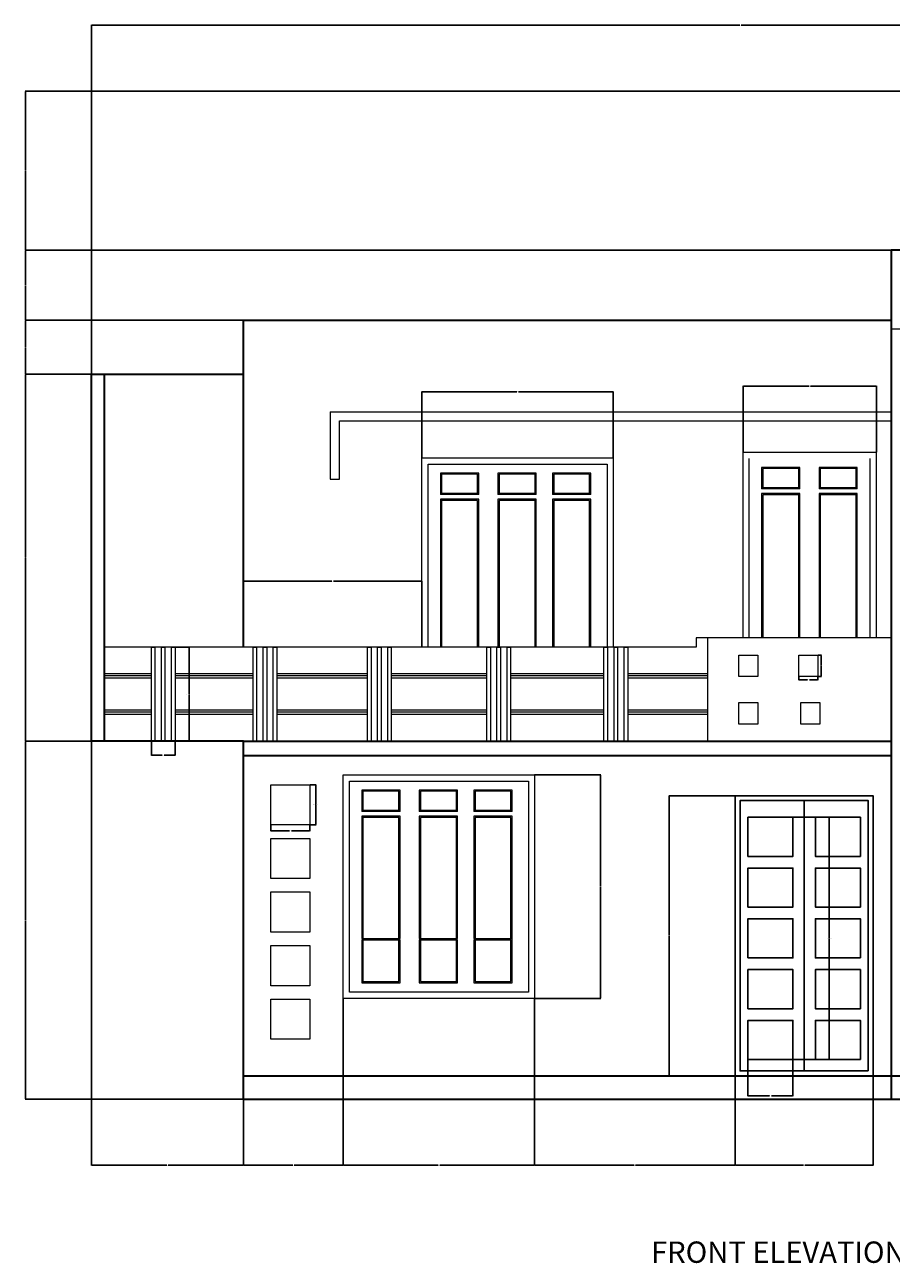
# Model space of a CAD drawing. Units: inches. Extents: x 1741 to 3812, y 9290 to 10023.
# Tile 4 of 5: x 3008 to 3495, y 9327 to 10023. Entities that reach past the tile are written whole.
import ezdxf

# ---------------------------------------------------------------- set-up
doc = ezdxf.new("R2010")
doc.units = ezdxf.units.IN
doc.header["$MEASUREMENT"] = 0
for name, color, linetype, lineweight in [('A-ANNO-DIMS', 2, 'Continuous', 18), ('A-ANNO-TEXT', 7, 'Continuous', 25), ('A-DOOR-ELEV', 3, 'Continuous', 25), ('A-ELEV', 7, 'Continuous', 35), ('A-ELEV-RAIL', 3, 'Continuous', 18), ('A-ELEV-TRIM', 9, 'Continuous', 18), ('A-GLAZ-ELEV', 4, 'Continuous', 18)]:
    doc.layers.add(name, color=color, linetype=linetype, lineweight=lineweight)
doc.styles.get("Standard").update_dxf_attribs({"font": 'arial.ttf'})
doc.dimstyles.get("Standard").update_dxf_attribs({"dimtxt": 0.18, "dimasz": 0.18, "dimexe": 0.18, "dimexo": 0.0625, "dimgap": 0.09, "dimtad": 0, "dimtih": 1, "dimtoh": 1, "dimdec": 4, "dimzin": 0, "dimdsep": 46, "dimtxsty": 'Standard', "dimcen": 0.09, "dimadec": 0, "dimazin": 0, "dimtfac": 1, "dimtdec": 4, "dimtofl": 0, "dimtmove": 0, "dimatfit": 3, "dimfxl": 1, "dimtolj": 1, "dimtzin": 0, "dimarcsym": 0})

# ---------------------------------------------------------------- blocks, each defined once
blk = doc.blocks.new('GLAZ-TRANSOM-LIGHT')
for p, q in [((0, 12.07), (0, 0)), ((21.51, 12.07), (0, 12.07)), ((0.66, 11.41), (0.66, 0.66)), ((20.85, 11.41), (0.66, 11.41)), ((20.85, 0.66), (20.85, 11.41)), ((21.51, 0), (21.51, 12.07)), ((20.85, 0.66), (0.66, 0.66)), ((21.51, 0), (0, 0))]:
    blk.add_line(p, q)
blk = doc.blocks.new('DOOR-LEAF-PANEL-SET')
for points in [[(0, 114.23), (25.3, 114.23), (25.3, 136.25), (0, 136.25)], [(0, 85.68), (25.3, 85.68), (25.3, 107.69), (0, 107.69)], [(0, 57.12), (25.3, 57.12), (25.3, 79.13), (0, 79.13)], [(0, 28.56), (25.3, 28.56), (25.3, 50.57), (0, 50.57)], [(0, 0), (25.3, 0), (25.3, 22.01), (0, 22.01)]]:
    blk.add_lwpolyline(points, close=True)
blk = doc.blocks.new('BALCONY-RAIL-POST-CLUSTER')
for points in [[(0, 52.73), (1.96, 52.73), (1.96, 0), (0, 0)], [(5.66, 52.73), (7.63, 52.73), (7.63, 0), (5.66, 0)], [(11.35, 52.73), (13.31, 52.73), (13.31, 0), (11.35, 0)]]:
    blk.add_lwpolyline(points, close=True)
blk = doc.blocks.new('BALCONY-PARAPET-REVEAL')
blk.add_lwpolyline([(0, 12.07), (10.64, 12.07), (10.64, 0), (0, 0)], close=True)
blk = doc.blocks.new('FACADE-RECESSED-PANEL')
blk.add_lwpolyline([(0, 22.57), (21.93, 22.57), (21.93, 0), (0, 0)], close=True)
blk = doc.blocks.new('*D19')
at = {"layer": 'A-ANNO-DIMS', "color": 0, "lineweight": -2, "transparency": 16777216}
for p, q in [((3092.52, 9673.01), (3100.55, 9673.01)), ((3100.37, 9672.83), (3100.37, 9646.83)), ((3100.37, 9620.47), (3100.37, 9646.47)), ((3092.52, 9620.29), (3100.55, 9620.29))]:
    blk.add_line(p, q, dxfattribs=at)
at = {"layer": 'A-ANNO-DIMS', "color": 0, "transparency": 16777216}
for points in [[(3100.34, 9672.83), (3100.4, 9672.83), (3100.37, 9673.01)], [(3100.34, 9620.47), (3100.4, 9620.47), (3100.37, 9620.29)]]:
    blk.add_solid(points, dxfattribs=at)
at = {"layer": 'Defpoints', "color": 0, "transparency": 16777216}
for p in [(3092.46, 9673.01), (3100.37, 9673.01), (3092.46, 9620.29)]:
    blk.add_point(p, dxfattribs=at)
at = {"layer": 'A-ANNO-DIMS', "color": 0, "transparency": 16777216, "insert": (3100.37, 9646.65), "char_height": 0.18, "attachment_point": 5}
blk.add_mtext('\\A1;RAIL POST GROUP 53 TYP.', dxfattribs=at)
blk = doc.blocks.new('*D20')
at = {"layer": 'A-ANNO-DIMS', "color": 0, "lineweight": -2, "transparency": 16777216}
for p, q in [((3079.15, 9620.22), (3079.15, 9612.2)), ((3092.46, 9620.22), (3092.46, 9612.2)), ((3079.33, 9612.38), (3085.29, 9612.38)), ((3092.28, 9612.38), (3086.33, 9612.38))]:
    blk.add_line(p, q, dxfattribs=at)
at = {"layer": 'A-ANNO-DIMS', "color": 0, "transparency": 16777216}
for points in [[(3079.33, 9612.41), (3079.33, 9612.35), (3079.15, 9612.38)], [(3092.28, 9612.41), (3092.28, 9612.35), (3092.46, 9612.38)]]:
    blk.add_solid(points, dxfattribs=at)
at = {"layer": 'Defpoints', "color": 0, "transparency": 16777216}
for p in [(3079.15, 9620.29), (3092.46, 9620.29), (3092.46, 9612.38)]:
    blk.add_point(p, dxfattribs=at)
at = {"layer": 'A-ANNO-DIMS', "color": 0, "transparency": 16777216, "insert": (3085.81, 9612.38), "char_height": 0.18, "attachment_point": 5}
blk.add_mtext('\\A1;13 TYP.', dxfattribs=at)
blk = doc.blocks.new('*D23')
at = {"layer": 'A-ANNO-DIMS', "color": 0, "lineweight": -2, "transparency": 16777216}
for p, q in [((3168.33, 9595.77), (3171.83, 9595.77)), ((3171.65, 9595.59), (3171.65, 9584.67)), ((3171.65, 9573.38), (3171.65, 9584.3)), ((3168.33, 9573.2), (3171.83, 9573.2))]:
    blk.add_line(p, q, dxfattribs=at)
at = {"layer": 'A-ANNO-DIMS', "color": 0, "transparency": 16777216}
for points in [[(3171.62, 9595.59), (3171.68, 9595.59), (3171.65, 9595.77)], [(3171.62, 9573.38), (3171.68, 9573.38), (3171.65, 9573.2)]]:
    blk.add_solid(points, dxfattribs=at)
at = {"layer": 'Defpoints', "color": 0, "transparency": 16777216}
for p in [(3168.27, 9595.77), (3171.65, 9595.77), (3168.27, 9573.2)]:
    blk.add_point(p, dxfattribs=at)
at = {"layer": 'A-ANNO-DIMS', "color": 0, "transparency": 16777216, "insert": (3171.65, 9584.48), "char_height": 0.18, "attachment_point": 5}
blk.add_mtext('\\A1;RECESSED PANEL 23 TYP.', dxfattribs=at)
blk = doc.blocks.new('*D24')
at = {"layer": 'A-ANNO-DIMS', "color": 0, "lineweight": -2, "transparency": 16777216}
for p, q in [((3146.33, 9573.14), (3146.33, 9569.63)), ((3168.27, 9573.14), (3168.27, 9569.63)), ((3146.51, 9569.81), (3156.77, 9569.81)), ((3168.09, 9569.81), (3157.83, 9569.81))]:
    blk.add_line(p, q, dxfattribs=at)
at = {"layer": 'A-ANNO-DIMS', "color": 0, "transparency": 16777216}
for points in [[(3146.51, 9569.84), (3146.51, 9569.78), (3146.33, 9569.81)], [(3168.09, 9569.84), (3168.09, 9569.78), (3168.27, 9569.81)]]:
    blk.add_solid(points, dxfattribs=at)
at = {"layer": 'Defpoints', "color": 0, "transparency": 16777216}
for p in [(3146.33, 9573.2), (3168.27, 9573.2), (3168.27, 9569.81)]:
    blk.add_point(p, dxfattribs=at)
at = {"layer": 'A-ANNO-DIMS', "color": 0, "transparency": 16777216, "insert": (3157.3, 9569.81), "char_height": 0.18, "attachment_point": 5}
blk.add_mtext('\\A1;22 TYP.', dxfattribs=at)
blk = doc.blocks.new('*D25')
at = {"layer": 'A-ANNO-DIMS', "color": 0, "lineweight": -2, "transparency": 16777216}
for p, q in [((3453.73, 9668.66), (3455.66, 9668.66)), ((3455.48, 9668.48), (3455.48, 9662.81)), ((3455.48, 9656.78), (3455.48, 9662.45)), ((3453.73, 9656.6), (3455.66, 9656.6))]:
    blk.add_line(p, q, dxfattribs=at)
at = {"layer": 'A-ANNO-DIMS', "color": 0, "transparency": 16777216}
for points in [[(3455.45, 9668.48), (3455.51, 9668.48), (3455.48, 9668.66)], [(3455.45, 9656.78), (3455.51, 9656.78), (3455.48, 9656.6)]]:
    blk.add_solid(points, dxfattribs=at)
at = {"layer": 'Defpoints', "color": 0, "transparency": 16777216}
for p in [(3453.67, 9668.66), (3455.48, 9668.66), (3453.67, 9656.6)]:
    blk.add_point(p, dxfattribs=at)
at = {"layer": 'A-ANNO-DIMS', "color": 0, "transparency": 16777216, "insert": (3455.48, 9662.63), "char_height": 0.18, "attachment_point": 5}
blk.add_mtext('\\A1;BALCONY REVEAL 12 TYP.', dxfattribs=at)
blk = doc.blocks.new('*D26')
at = {"layer": 'A-ANNO-DIMS', "color": 0, "lineweight": -2, "transparency": 16777216}
for p, q in [((3443.02, 9656.54), (3443.02, 9654.61)), ((3453.67, 9656.54), (3453.67, 9654.61)), ((3443.2, 9654.79), (3447.82, 9654.79)), ((3453.49, 9654.79), (3448.86, 9654.79))]:
    blk.add_line(p, q, dxfattribs=at)
at = {"layer": 'A-ANNO-DIMS', "color": 0, "transparency": 16777216}
for points in [[(3443.2, 9654.82), (3443.2, 9654.76), (3443.02, 9654.79)], [(3453.49, 9654.82), (3453.49, 9654.76), (3453.67, 9654.79)]]:
    blk.add_solid(points, dxfattribs=at)
at = {"layer": 'Defpoints', "color": 0, "transparency": 16777216}
for p in [(3443.02, 9656.6), (3453.67, 9656.6), (3453.67, 9654.79)]:
    blk.add_point(p, dxfattribs=at)
at = {"layer": 'A-ANNO-DIMS', "color": 0, "transparency": 16777216, "insert": (3448.34, 9654.79), "char_height": 0.18, "attachment_point": 5}
blk.add_mtext('\\A1;11 TYP.', dxfattribs=at)
blk = doc.blocks.new('*D29')
at = {"layer": 'A-ANNO-DIMS', "color": 0, "lineweight": -2, "transparency": 16777216}
for p, q in [((3439.68, 9577.53), (3460.23, 9577.53)), ((3460.05, 9577.35), (3460.05, 9509.59)), ((3460.05, 9441.46), (3460.05, 9509.22)), ((3439.68, 9441.28), (3460.23, 9441.28))]:
    blk.add_line(p, q, dxfattribs=at)
at = {"layer": 'A-ANNO-DIMS', "color": 0, "transparency": 16777216}
for points in [[(3460.02, 9577.35), (3460.08, 9577.35), (3460.05, 9577.53)], [(3460.02, 9441.46), (3460.08, 9441.46), (3460.05, 9441.28)]]:
    blk.add_solid(points, dxfattribs=at)
at = {"layer": 'Defpoints', "color": 0, "transparency": 16777216}
for p in [(3439.61, 9577.53), (3460.05, 9577.53), (3439.61, 9441.28)]:
    blk.add_point(p, dxfattribs=at)
at = {"layer": 'A-ANNO-DIMS', "color": 0, "transparency": 16777216, "insert": (3460.05, 9509.41), "char_height": 0.18, "attachment_point": 5}
blk.add_mtext('\\A1;LEAF PANELS 136 TYP.', dxfattribs=at)
blk = doc.blocks.new('*D30')
at = {"layer": 'A-ANNO-DIMS', "color": 0, "lineweight": -2, "transparency": 16777216}
for p, q in [((3414.31, 9441.22), (3414.31, 9420.66)), ((3439.61, 9441.22), (3439.61, 9420.66)), ((3414.49, 9420.84), (3426.43, 9420.84)), ((3439.43, 9420.84), (3427.49, 9420.84))]:
    blk.add_line(p, q, dxfattribs=at)
at = {"layer": 'A-ANNO-DIMS', "color": 0, "transparency": 16777216}
for points in [[(3414.49, 9420.87), (3414.49, 9420.81), (3414.31, 9420.84)], [(3439.43, 9420.87), (3439.43, 9420.81), (3439.61, 9420.84)]]:
    blk.add_solid(points, dxfattribs=at)
at = {"layer": 'Defpoints', "color": 0, "transparency": 16777216}
for p in [(3414.31, 9441.28), (3439.61, 9441.28), (3439.61, 9420.84)]:
    blk.add_point(p, dxfattribs=at)
at = {"layer": 'A-ANNO-DIMS', "color": 0, "transparency": 16777216, "insert": (3426.96, 9420.84), "char_height": 0.18, "attachment_point": 5}
blk.add_mtext('\\A1;25 TYP.', dxfattribs=at)
blk = doc.blocks.new('*D77')
at = {"layer": 'A-ANNO-DIMS', "color": 0, "lineweight": -2, "transparency": 16777216}
for p, q in [((3045.51, 9826.55), (3045.51, 10022.94)), ((3045.69, 10022.76), (3409.82, 10022.76)), ((3774.74, 10022.76), (3410.61, 10022.76)), ((3774.92, 9985.72), (3774.92, 10022.94))]:
    blk.add_line(p, q, dxfattribs=at)
at = {"layer": 'A-ANNO-DIMS', "color": 0, "transparency": 16777216}
for points in [[(3045.69, 10022.79), (3045.69, 10022.73), (3045.51, 10022.76)], [(3774.74, 10022.79), (3774.74, 10022.73), (3774.92, 10022.76)]]:
    blk.add_solid(points, dxfattribs=at)
at = {"layer": 'Defpoints', "color": 0, "transparency": 16777216}
for p in [(3774.92, 10022.76), (3774.92, 9985.66), (3045.51, 9826.49)]:
    blk.add_point(p, dxfattribs=at)
at = {"layer": 'A-ANNO-DIMS', "color": 0, "transparency": 16777216, "insert": (3410.21, 10022.76), "char_height": 0.18, "attachment_point": 5}
blk.add_mtext('\\A1;729.4', dxfattribs=at)
blk = doc.blocks.new('*D79')
at = {"layer": 'A-ANNO-DIMS', "color": 0, "lineweight": -2, "transparency": 16777216}
for p, q in [((3045.51, 9620.22), (3045.51, 9381.78)), ((3130.92, 9419), (3130.92, 9381.78)), ((3045.69, 9381.96), (3087.89, 9381.96)), ((3130.74, 9381.96), (3088.54, 9381.96))]:
    blk.add_line(p, q, dxfattribs=at)
at = {"layer": 'A-ANNO-DIMS', "color": 0, "transparency": 16777216}
for points in [[(3045.69, 9381.99), (3045.69, 9381.93), (3045.51, 9381.96)], [(3130.74, 9381.99), (3130.74, 9381.93), (3130.92, 9381.96)]]:
    blk.add_solid(points, dxfattribs=at)
at = {"layer": 'Defpoints', "color": 0, "transparency": 16777216}
for p in [(3045.51, 9620.29), (3130.92, 9419.06), (3130.92, 9381.96)]:
    blk.add_point(p, dxfattribs=at)
at = {"layer": 'A-ANNO-DIMS', "color": 0, "transparency": 16777216, "insert": (3088.22, 9381.96), "char_height": 0.18, "attachment_point": 5}
blk.add_mtext('\\A1;85.4', dxfattribs=at)
blk = doc.blocks.new('*D80')
at = {"layer": 'A-ANNO-DIMS', "color": 0, "lineweight": -2, "transparency": 16777216}
for p, q in [((3186.98, 9475.64), (3186.98, 9381.78)), ((3130.92, 9419), (3130.92, 9381.78)), ((3131.1, 9381.96), (3158.56, 9381.96)), ((3186.8, 9381.96), (3159.34, 9381.96))]:
    blk.add_line(p, q, dxfattribs=at)
at = {"layer": 'A-ANNO-DIMS', "color": 0, "transparency": 16777216}
for points in [[(3131.1, 9381.99), (3131.1, 9381.93), (3130.92, 9381.96)], [(3186.8, 9381.99), (3186.8, 9381.93), (3186.98, 9381.96)]]:
    blk.add_solid(points, dxfattribs=at)
at = {"layer": 'Defpoints', "color": 0, "transparency": 16777216}
for p in [(3186.98, 9475.7), (3130.92, 9419.06), (3186.98, 9381.96)]:
    blk.add_point(p, dxfattribs=at)
at = {"layer": 'A-ANNO-DIMS', "color": 0, "transparency": 16777216, "insert": (3158.95, 9381.96), "char_height": 0.18, "attachment_point": 5}
blk.add_mtext('\\A1;56.07', dxfattribs=at)
blk = doc.blocks.new('*D81')
at = {"layer": 'A-ANNO-DIMS', "color": 0, "lineweight": -2, "transparency": 16777216}
for p, q in [((3186.98, 9475.64), (3186.98, 9381.78)), ((3294.43, 9475.64), (3294.43, 9381.78)), ((3187.16, 9381.96), (3240.25, 9381.96)), ((3294.25, 9381.96), (3241.16, 9381.96))]:
    blk.add_line(p, q, dxfattribs=at)
at = {"layer": 'A-ANNO-DIMS', "color": 0, "transparency": 16777216}
for points in [[(3187.16, 9381.99), (3187.16, 9381.93), (3186.98, 9381.96)], [(3294.25, 9381.99), (3294.25, 9381.93), (3294.43, 9381.96)]]:
    blk.add_solid(points, dxfattribs=at)
at = {"layer": 'Defpoints', "color": 0, "transparency": 16777216}
for p in [(3186.98, 9475.7), (3294.43, 9475.7), (3294.43, 9381.96)]:
    blk.add_point(p, dxfattribs=at)
at = {"layer": 'A-ANNO-DIMS', "color": 0, "transparency": 16777216, "insert": (3240.71, 9381.96), "char_height": 0.18, "attachment_point": 5}
blk.add_mtext('\\A1;107.44', dxfattribs=at)
blk = doc.blocks.new('*D82')
at = {"layer": 'A-ANNO-DIMS', "color": 0, "lineweight": -2, "transparency": 16777216}
for p, q in [((3294.43, 9475.64), (3294.43, 9381.78)), ((3407.19, 9432.13), (3407.19, 9381.78)), ((3294.61, 9381.96), (3350.35, 9381.96)), ((3407.01, 9381.96), (3351.26, 9381.96))]:
    blk.add_line(p, q, dxfattribs=at)
at = {"layer": 'A-ANNO-DIMS', "color": 0, "transparency": 16777216}
for points in [[(3294.61, 9381.99), (3294.61, 9381.93), (3294.43, 9381.96)], [(3407.01, 9381.99), (3407.01, 9381.93), (3407.19, 9381.96)]]:
    blk.add_solid(points, dxfattribs=at)
at = {"layer": 'Defpoints', "color": 0, "transparency": 16777216}
for p in [(3294.43, 9475.7), (3407.19, 9432.19), (3407.19, 9381.96)]:
    blk.add_point(p, dxfattribs=at)
at = {"layer": 'A-ANNO-DIMS', "color": 0, "transparency": 16777216, "insert": (3350.81, 9381.96), "char_height": 0.18, "attachment_point": 5}
blk.add_mtext('\\A1;112.76', dxfattribs=at)
blk = doc.blocks.new('*D83')
at = {"layer": 'A-ANNO-DIMS', "color": 0, "lineweight": -2, "transparency": 16777216}
for p, q in [((3407.19, 9432.13), (3407.19, 9381.78)), ((3484.64, 9432.13), (3484.64, 9381.78)), ((3407.37, 9381.96), (3445.52, 9381.96)), ((3484.46, 9381.96), (3446.31, 9381.96))]:
    blk.add_line(p, q, dxfattribs=at)
at = {"layer": 'A-ANNO-DIMS', "color": 0, "transparency": 16777216}
for points in [[(3407.37, 9381.99), (3407.37, 9381.93), (3407.19, 9381.96)], [(3484.46, 9381.99), (3484.46, 9381.93), (3484.64, 9381.96)]]:
    blk.add_solid(points, dxfattribs=at)
at = {"layer": 'Defpoints', "color": 0, "transparency": 16777216}
for p in [(3407.19, 9432.19), (3484.64, 9432.19), (3484.64, 9381.96)]:
    blk.add_point(p, dxfattribs=at)
at = {"layer": 'A-ANNO-DIMS', "color": 0, "transparency": 16777216, "insert": (3445.92, 9381.96), "char_height": 0.18, "attachment_point": 5}
blk.add_mtext('\\A1;77.46', dxfattribs=at)
blk = doc.blocks.new('*D87')
at = {"layer": 'A-ANNO-DIMS', "color": 0, "lineweight": -2, "transparency": 16777216}
for p, q in [((3130.86, 9620.29), (3008.23, 9620.29)), ((3008.41, 9620.11), (3008.41, 9519.86)), ((3008.41, 9419.24), (3008.41, 9519.49)), ((3130.86, 9419.06), (3008.23, 9419.06))]:
    blk.add_line(p, q, dxfattribs=at)
at = {"layer": 'A-ANNO-DIMS', "color": 0, "transparency": 16777216}
for points in [[(3008.38, 9620.11), (3008.44, 9620.11), (3008.41, 9620.29)], [(3008.38, 9419.24), (3008.44, 9419.24), (3008.41, 9419.06)]]:
    blk.add_solid(points, dxfattribs=at)
at = {"layer": 'Defpoints', "color": 0, "transparency": 16777216}
for p in [(3008.41, 9620.29), (3130.92, 9620.29), (3130.92, 9419.06)]:
    blk.add_point(p, dxfattribs=at)
at = {"layer": 'A-ANNO-DIMS', "color": 0, "transparency": 16777216, "insert": (3008.41, 9519.67), "char_height": 0.18, "attachment_point": 5}
blk.add_mtext('\\A1;201.23', dxfattribs=at)
blk = doc.blocks.new('*D88')
at = {"layer": 'A-ANNO-DIMS', "color": 0, "lineweight": -2, "transparency": 16777216}
for p, q in [((3045.45, 9826.49), (3008.23, 9826.49)), ((3008.41, 9826.31), (3008.41, 9723.57)), ((3008.41, 9620.47), (3008.41, 9723.21)), ((3045.45, 9620.29), (3008.23, 9620.29))]:
    blk.add_line(p, q, dxfattribs=at)
at = {"layer": 'A-ANNO-DIMS', "color": 0, "transparency": 16777216}
for points in [[(3008.38, 9826.31), (3008.44, 9826.31), (3008.41, 9826.49)], [(3008.38, 9620.47), (3008.44, 9620.47), (3008.41, 9620.29)]]:
    blk.add_solid(points, dxfattribs=at)
at = {"layer": 'Defpoints', "color": 0, "transparency": 16777216}
for p in [(3008.41, 9826.49), (3045.51, 9826.49), (3045.51, 9620.29)]:
    blk.add_point(p, dxfattribs=at)
at = {"layer": 'A-ANNO-DIMS', "color": 0, "transparency": 16777216, "insert": (3008.41, 9723.39), "char_height": 0.18, "attachment_point": 5}
blk.add_mtext('\\A1;206.2', dxfattribs=at)
blk = doc.blocks.new('*D89')
at = {"layer": 'A-ANNO-DIMS', "color": 0, "lineweight": -2, "transparency": 16777216}
for p, q in [((3130.86, 9856.96), (3008.23, 9856.96)), ((3008.41, 9856.78), (3008.41, 9841.91)), ((3008.41, 9826.67), (3008.41, 9841.54)), ((3045.45, 9826.49), (3008.23, 9826.49))]:
    blk.add_line(p, q, dxfattribs=at)
at = {"layer": 'A-ANNO-DIMS', "color": 0, "transparency": 16777216}
for points in [[(3008.38, 9856.78), (3008.44, 9856.78), (3008.41, 9856.96)], [(3008.38, 9826.67), (3008.44, 9826.67), (3008.41, 9826.49)]]:
    blk.add_solid(points, dxfattribs=at)
at = {"layer": 'Defpoints', "color": 0, "transparency": 16777216}
for p in [(3008.41, 9856.96), (3130.92, 9856.96), (3045.51, 9826.49)]:
    blk.add_point(p, dxfattribs=at)
at = {"layer": 'A-ANNO-DIMS', "color": 0, "transparency": 16777216, "insert": (3008.41, 9841.73), "char_height": 0.18, "attachment_point": 5}
blk.add_mtext('\\A1;30.47', dxfattribs=at)
blk = doc.blocks.new('*D90')
at = {"layer": 'A-ANNO-DIMS', "color": 0, "lineweight": -2, "transparency": 16777216}
for p, q in [((3494.79, 9896.18), (3008.23, 9896.18)), ((3008.41, 9896), (3008.41, 9876.75)), ((3008.41, 9857.14), (3008.41, 9876.39)), ((3130.86, 9856.96), (3008.23, 9856.96))]:
    blk.add_line(p, q, dxfattribs=at)
at = {"layer": 'A-ANNO-DIMS', "color": 0, "transparency": 16777216}
for points in [[(3008.38, 9896), (3008.44, 9896), (3008.41, 9896.18)], [(3008.38, 9857.14), (3008.44, 9857.14), (3008.41, 9856.96)]]:
    blk.add_solid(points, dxfattribs=at)
at = {"layer": 'Defpoints', "color": 0, "transparency": 16777216}
for p in [(3008.41, 9896.18), (3494.85, 9896.18), (3130.92, 9856.96)]:
    blk.add_point(p, dxfattribs=at)
at = {"layer": 'A-ANNO-DIMS', "color": 0, "transparency": 16777216, "insert": (3008.41, 9876.57), "char_height": 0.18, "attachment_point": 5}
blk.add_mtext('\\A1;39.22', dxfattribs=at)
blk = doc.blocks.new('*D91')
at = {"layer": 'A-ANNO-DIMS', "color": 0, "lineweight": -2, "transparency": 16777216}
for p, q in [((3580.43, 9985.66), (3008.23, 9985.66)), ((3008.41, 9985.48), (3008.41, 9941.1)), ((3008.41, 9896.36), (3008.41, 9940.74)), ((3494.79, 9896.18), (3008.23, 9896.18))]:
    blk.add_line(p, q, dxfattribs=at)
at = {"layer": 'A-ANNO-DIMS', "color": 0, "transparency": 16777216}
for points in [[(3008.38, 9985.48), (3008.44, 9985.48), (3008.41, 9985.66)], [(3008.38, 9896.36), (3008.44, 9896.36), (3008.41, 9896.18)]]:
    blk.add_solid(points, dxfattribs=at)
at = {"layer": 'Defpoints', "color": 0, "transparency": 16777216}
for p in [(3008.41, 9985.66), (3580.49, 9985.66), (3494.85, 9896.18)]:
    blk.add_point(p, dxfattribs=at)
at = {"layer": 'A-ANNO-DIMS', "color": 0, "transparency": 16777216, "insert": (3008.41, 9940.92), "char_height": 0.18, "attachment_point": 5}
blk.add_mtext('\\A1;89.48', dxfattribs=at)
blk = doc.blocks.new('*D94')
at = {"layer": 'A-ANNO-DIMS', "color": 0, "lineweight": -2, "transparency": 16777216}
for p, q in [((3294.49, 9601.3), (3331.71, 9601.3)), ((3331.53, 9601.12), (3331.53, 9538.68)), ((3331.53, 9475.88), (3331.53, 9538.32)), ((3294.49, 9475.7), (3331.71, 9475.7))]:
    blk.add_line(p, q, dxfattribs=at)
at = {"layer": 'A-ANNO-DIMS', "color": 0, "transparency": 16777216}
for points in [[(3331.5, 9601.12), (3331.56, 9601.12), (3331.53, 9601.3)], [(3331.5, 9475.88), (3331.56, 9475.88), (3331.53, 9475.7)]]:
    blk.add_solid(points, dxfattribs=at)
at = {"layer": 'Defpoints', "color": 0, "transparency": 16777216}
for p in [(3294.43, 9601.3), (3294.43, 9475.7), (3331.53, 9475.7)]:
    blk.add_point(p, dxfattribs=at)
at = {"layer": 'A-ANNO-DIMS', "color": 0, "transparency": 16777216, "insert": (3331.53, 9538.5), "char_height": 0.18, "attachment_point": 5}
blk.add_mtext('\\A1;125.6', dxfattribs=at)
blk = doc.blocks.new('*D95')
at = {"layer": 'A-ANNO-DIMS', "color": 0, "lineweight": -2, "transparency": 16777216}
for p, q in [((3407.13, 9589.56), (3369.91, 9589.56)), ((3370.09, 9589.38), (3370.09, 9511.06)), ((3370.09, 9432.37), (3370.09, 9510.69)), ((3407.13, 9432.19), (3369.91, 9432.19))]:
    blk.add_line(p, q, dxfattribs=at)
at = {"layer": 'A-ANNO-DIMS', "color": 0, "transparency": 16777216}
for points in [[(3370.06, 9589.38), (3370.12, 9589.38), (3370.09, 9589.56)], [(3370.06, 9432.37), (3370.12, 9432.37), (3370.09, 9432.19)]]:
    blk.add_solid(points, dxfattribs=at)
at = {"layer": 'Defpoints', "color": 0, "transparency": 16777216}
for p in [(3370.09, 9589.56), (3407.19, 9589.56), (3407.19, 9432.19)]:
    blk.add_point(p, dxfattribs=at)
at = {"layer": 'A-ANNO-DIMS', "color": 0, "transparency": 16777216, "insert": (3370.09, 9510.87), "char_height": 0.18, "attachment_point": 5}
blk.add_mtext('\\A1;157.36', dxfattribs=at)
blk = doc.blocks.new('*D98')
at = {"layer": 'A-ANNO-DIMS', "color": 0, "lineweight": -2, "transparency": 16777216}
for p, q in [((3130.92, 9673.08), (3130.92, 9710.29)), ((3131.1, 9710.11), (3180.59, 9710.11)), ((3230.99, 9710.11), (3181.5, 9710.11)), ((3231.17, 9673.08), (3231.17, 9710.29))]:
    blk.add_line(p, q, dxfattribs=at)
at = {"layer": 'A-ANNO-DIMS', "color": 0, "transparency": 16777216}
for points in [[(3131.1, 9710.14), (3131.1, 9710.08), (3130.92, 9710.11)], [(3230.99, 9710.14), (3230.99, 9710.08), (3231.17, 9710.11)]]:
    blk.add_solid(points, dxfattribs=at)
at = {"layer": 'Defpoints', "color": 0, "transparency": 16777216}
for p in [(3231.17, 9710.11), (3130.92, 9673.01), (3231.17, 9673.01)]:
    blk.add_point(p, dxfattribs=at)
at = {"layer": 'A-ANNO-DIMS', "color": 0, "transparency": 16777216, "insert": (3181.05, 9710.11), "char_height": 0.18, "attachment_point": 5}
blk.add_mtext('\\A1;100.25', dxfattribs=at)
blk = doc.blocks.new('*D99')
at = {"layer": 'A-ANNO-DIMS', "color": 0, "lineweight": -2, "transparency": 16777216}
for p, q in [((3231.17, 9779.53), (3231.17, 9816.75)), ((3231.35, 9816.57), (3284.44, 9816.57)), ((3338.44, 9816.57), (3285.35, 9816.57)), ((3338.62, 9779.53), (3338.62, 9816.75))]:
    blk.add_line(p, q, dxfattribs=at)
at = {"layer": 'A-ANNO-DIMS', "color": 0, "transparency": 16777216}
for points in [[(3231.35, 9816.6), (3231.35, 9816.54), (3231.17, 9816.57)], [(3338.44, 9816.6), (3338.44, 9816.54), (3338.62, 9816.57)]]:
    blk.add_solid(points, dxfattribs=at)
at = {"layer": 'Defpoints', "color": 0, "transparency": 16777216}
for p in [(3338.62, 9816.57), (3231.17, 9779.47), (3338.62, 9779.47)]:
    blk.add_point(p, dxfattribs=at)
at = {"layer": 'A-ANNO-DIMS', "color": 0, "transparency": 16777216, "insert": (3284.89, 9816.57), "char_height": 0.18, "attachment_point": 5}
blk.add_mtext('\\A1;107.44', dxfattribs=at)
blk = doc.blocks.new('*D100')
at = {"layer": 'A-ANNO-DIMS', "color": 0, "lineweight": -2, "transparency": 16777216}
for p, q in [((3411.6, 9782.71), (3411.6, 9819.93)), ((3411.78, 9819.75), (3448.68, 9819.75)), ((3486.36, 9819.75), (3449.47, 9819.75)), ((3486.54, 9782.71), (3486.54, 9819.93))]:
    blk.add_line(p, q, dxfattribs=at)
at = {"layer": 'A-ANNO-DIMS', "color": 0, "transparency": 16777216}
for points in [[(3411.78, 9819.78), (3411.78, 9819.72), (3411.6, 9819.75)], [(3486.36, 9819.78), (3486.36, 9819.72), (3486.54, 9819.75)]]:
    blk.add_solid(points, dxfattribs=at)
at = {"layer": 'Defpoints', "color": 0, "transparency": 16777216}
for p in [(3486.54, 9819.75), (3411.6, 9782.65), (3486.54, 9782.65)]:
    blk.add_point(p, dxfattribs=at)
at = {"layer": 'A-ANNO-DIMS', "color": 0, "transparency": 16777216, "insert": (3449.07, 9819.75), "char_height": 0.18, "attachment_point": 5}
blk.add_mtext('\\A1;74.94', dxfattribs=at)

msp = doc.modelspace()

# ---------------------------------------------------------------- linework, layer by layer
at = {"layer": 'A-DOOR-ELEV'}
msp.add_line((3445.916, 9434.8933), (3445.916, 9586.8566), dxfattribs=at)
for points in [[(3484.6443, 9432.1944), (3407.1877, 9432.1944), (3407.1877, 9589.5555), (3484.6443, 9589.5555)], [(3481.9454, 9434.8933), (3409.8866, 9434.8933), (3409.8866, 9586.8566), (3481.9454, 9586.8566)]]:
    msp.add_lwpolyline(points, close=True, dxfattribs=at)
at = {"layer": 'A-ELEV'}
for p, q in [((3774.9155, 9896.1797), (3494.8475, 9896.1797)), ((3494.8475, 9896.1797), (3494.8475, 9419.0599)), ((3130.9182, 9856.9629), (3494.8475, 9856.9629)), ((3130.9182, 9673.0135), (3130.9182, 9856.9629)), ((3045.5138, 9620.287), (3045.5138, 9826.4899)), ((3045.5138, 9826.4899), (3130.9182, 9826.4899)), ((3052.8477, 9620.287), (3052.8477, 9826.4899)), ((3130.9182, 9620.287), (3045.5138, 9620.287)), ((3130.9182, 9620.287), (3494.8475, 9620.287)), ((3130.9182, 9419.0599), (3130.9182, 9620.287)), ((3130.9182, 9612.1944), (3494.8475, 9612.1944)), ((3130.9182, 9432.1944), (3774.9155, 9432.1944)), ((3130.9182, 9419.0599), (3774.9155, 9419.0599))]:
    msp.add_line(p, q, dxfattribs=at)
at = {"layer": 'A-ELEV-RAIL'}
for p, q in [((3494.8475, 9678.3912), (3385.1873, 9678.3912)), ((3385.1873, 9678.3912), (3385.1873, 9673.0135)), ((3391.6128, 9678.3912), (3391.6128, 9620.287)), ((3385.1873, 9673.0135), (3052.8477, 9673.0135)), ((3052.8477, 9658.2536), (3079.1511, 9658.2536)), ((3052.8477, 9657.0864), (3079.1511, 9657.0864)), ((3052.8477, 9655.9193), (3079.1511, 9655.9193)), ((3092.4615, 9658.2536), (3136.3361, 9658.2536)), ((3092.4615, 9657.0864), (3136.3361, 9657.0864)), ((3092.4615, 9655.9193), (3136.3361, 9655.9193)), ((3149.6465, 9658.2536), (3200.6041, 9658.2536)), ((3149.6465, 9657.0864), (3200.6041, 9657.0864)), ((3149.6465, 9655.9193), (3200.6041, 9655.9193)), ((3213.9145, 9658.2536), (3267.6685, 9658.2536)), ((3213.9145, 9657.0864), (3267.6685, 9657.0864)), ((3213.9145, 9655.9193), (3267.6685, 9655.9193)), ((3280.9789, 9658.2536), (3333.461, 9658.2536)), ((3280.9789, 9657.0864), (3333.461, 9657.0864)), ((3280.9789, 9655.9193), (3333.461, 9655.9193)), ((3346.7714, 9658.2536), (3391.6128, 9658.2536)), ((3346.7714, 9657.0864), (3391.6128, 9657.0864)), ((3346.7714, 9655.9193), (3391.6128, 9655.9193)), ((3052.8477, 9637.8286), (3079.1511, 9637.8286)), ((3052.8477, 9636.6615), (3079.1511, 9636.6615)), ((3052.8477, 9635.4943), (3079.1511, 9635.4943)), ((3092.4615, 9637.8286), (3136.3361, 9637.8286)), ((3092.4615, 9636.6615), (3136.3361, 9636.6615)), ((3092.4615, 9635.4943), (3136.3361, 9635.4943)), ((3149.6465, 9637.8286), (3200.6041, 9637.8286)), ((3149.6465, 9636.6615), (3200.6041, 9636.6615)), ((3149.6465, 9635.4943), (3200.6041, 9635.4943)), ((3213.9145, 9637.8286), (3267.6685, 9637.8286)), ((3213.9145, 9636.6615), (3267.6685, 9636.6615)), ((3213.9145, 9635.4943), (3267.6685, 9635.4943)), ((3280.9789, 9637.8286), (3333.461, 9637.8286)), ((3280.9789, 9636.6615), (3333.461, 9636.6615)), ((3280.9789, 9635.4943), (3333.461, 9635.4943)), ((3346.7714, 9637.8286), (3391.6128, 9637.8286)), ((3346.7714, 9636.6615), (3391.6128, 9636.6615)), ((3346.7714, 9635.4943), (3391.6128, 9635.4943))]:
    msp.add_line(p, q, dxfattribs=at)
msp.add_lwpolyline([(3338.6172, 9620.287), (3231.1727, 9620.287)], dxfattribs=at)
at = {"layer": 'A-ELEV-TRIM'}
for p, q in [((3730.5782, 9851.7953), (3494.8475, 9851.7953)), ((3179.5944, 9805.3348), (3494.8475, 9805.3348)), ((3179.5944, 9805.3348), (3179.5944, 9767.4573)), ((3184.8682, 9800.287), (3494.8475, 9800.287)), ((3184.8682, 9767.4573), (3184.8682, 9800.287)), ((3179.5944, 9767.4573), (3184.8682, 9767.4573))]:
    msp.add_line(p, q, dxfattribs=at)
at = {"layer": 'A-GLAZ-ELEV'}
for p, q in [((3411.6009, 9782.6524), (3486.5446, 9782.6524)), ((3263.1033, 9756.2208), (3241.5898, 9756.2208)), ((3241.5898, 9756.2208), (3241.5898, 9673.0135)), ((3262.4415, 9755.5591), (3242.2515, 9755.5591)), ((3242.2515, 9755.5591), (3242.2515, 9673.0135)), ((3262.4415, 9673.0135), (3262.4415, 9755.5591)), ((3263.1033, 9673.0135), (3263.1033, 9756.2208)), ((3443.5315, 9759.4078), (3422.018, 9759.4078)), ((3422.018, 9759.4078), (3422.018, 9678.3912)), ((3442.8697, 9758.7461), (3422.6797, 9758.7461)), ((3422.6797, 9758.7461), (3422.6797, 9678.3912)), ((3442.8697, 9678.3912), (3442.8697, 9758.7461)), ((3443.5315, 9678.3912), (3443.5315, 9759.4078)), ((3218.9149, 9578.0555), (3197.4014, 9578.0555)), ((3197.4014, 9578.0555), (3197.4014, 9509.2975)), ((3218.2531, 9577.3937), (3198.0631, 9577.3937)), ((3198.0631, 9577.3937), (3198.0631, 9509.2975)), ((3218.2531, 9509.2975), (3218.2531, 9577.3937)), ((3218.9149, 9509.2975), (3218.9149, 9578.0555)), ((3197.4014, 9509.2975), (3218.9149, 9509.2975)), ((3229.6716, 9509.2975), (3251.1851, 9509.2975)), ((3260.3482, 9509.2975), (3281.8616, 9509.2975)), ((3197.4014, 9508.6357), (3218.9149, 9508.6357)), ((3197.4014, 9508.6357), (3197.4014, 9484.5013)), ((3198.0631, 9508.6357), (3198.0631, 9485.163)), ((3218.2531, 9485.163), (3218.2531, 9508.6357)), ((3218.9149, 9484.5013), (3218.9149, 9508.6357)), ((3229.6716, 9508.6357), (3251.1851, 9508.6357)), ((3260.3482, 9508.6357), (3281.1999, 9508.6357)), ((3197.4014, 9484.5013), (3218.9149, 9484.5013)), ((3198.0631, 9485.163), (3218.2531, 9485.163))]:
    msp.add_line(p, q, dxfattribs=at)
for points in [[(3411.6009, 9678.3912), (3411.6009, 9782.6524)], [(3486.5446, 9678.3912), (3486.5446, 9782.6524)], [(3231.1727, 9673.0135), (3231.1727, 9779.4654), (3338.6172, 9779.4654), (3338.6172, 9673.0135)], [(3234.609, 9673.0135), (3234.609, 9776.0292), (3335.181, 9776.0292), (3335.181, 9673.0135)], [(3415.0372, 9678.3912), (3415.0372, 9779.2162)], [(3483.1083, 9678.3912), (3483.1083, 9779.2162)], [(3295.3735, 9673.0135), (3295.3735, 9756.2208), (3273.86, 9756.2208), (3273.86, 9673.0135)], [(3294.7117, 9673.0135), (3294.7117, 9755.5591), (3274.5218, 9755.5591), (3274.5218, 9673.0135)], [(3326.05, 9673.0135), (3326.05, 9756.2208), (3304.5366, 9756.2208), (3304.5366, 9673.0135)], [(3325.3883, 9673.0135), (3325.3883, 9755.5591), (3305.1983, 9755.5591), (3305.1983, 9673.0135)], [(3475.8017, 9678.3912), (3475.8017, 9759.4078), (3454.2882, 9759.4078), (3454.2882, 9678.3912)], [(3475.1399, 9678.3912), (3475.1399, 9758.7461), (3454.95, 9758.7461), (3454.95, 9678.3912)], [(3251.1851, 9509.2975), (3251.1851, 9578.0555), (3229.6716, 9578.0555), (3229.6716, 9509.2975)], [(3250.5233, 9509.2975), (3250.5233, 9577.3937), (3230.3333, 9577.3937), (3230.3333, 9509.2975)], [(3260.3482, 9508.6357), (3260.3482, 9484.5013), (3281.8616, 9484.5013), (3281.8616, 9578.0555), (3260.3482, 9578.0555), (3260.3482, 9509.2975)], [(3281.1999, 9509.2975), (3281.1999, 9577.3937), (3261.0099, 9577.3937), (3261.0099, 9509.2975)], [(3229.6716, 9508.6357), (3229.6716, 9484.5013), (3251.1851, 9484.5013), (3251.1851, 9508.6357)], [(3230.3333, 9508.6357), (3230.3333, 9485.163), (3250.5233, 9485.163), (3250.5233, 9508.6357)], [(3261.0099, 9508.6357), (3261.0099, 9485.163), (3281.1999, 9485.163), (3281.1999, 9508.6357)]]:
    msp.add_lwpolyline(points, dxfattribs=at)
for points in [[(3186.9843, 9601.3001), (3294.4288, 9601.3001), (3294.4288, 9475.7043), (3186.9843, 9475.7043)], [(3190.4206, 9597.8638), (3290.9926, 9597.8638), (3290.9926, 9479.1406), (3190.4206, 9479.1406)]]:
    msp.add_lwpolyline(points, close=True, dxfattribs=at)

# ---------------------------------------------------------------- block references
at = {"layer": 'A-DOOR-ELEV'}
msp.add_blockref('DOOR-LEAF-PANEL-SET', (3414.309, 9441.282), dxfattribs=at)
at = {"layer": 'A-DOOR-ELEV', "extrusion": (0, 0, -1), "zscale": -1}
msp.add_blockref('DOOR-LEAF-PANEL-SET', (-3477.523, 9441.282), dxfattribs=at)
at = {"layer": 'A-ELEV-RAIL'}
for p in [(3079.151, 9620.287), (3136.336, 9620.287), (3200.6039, 9620.287), (3267.6684, 9620.287), (3333.4609, 9620.287)]:
    msp.add_blockref('BALCONY-RAIL-POST-CLUSTER', p, dxfattribs=at)
at = {"layer": 'A-ELEV-TRIM'}
for name, p in [('BALCONY-PARAPET-REVEAL', (3409.251, 9656.598)), ('BALCONY-PARAPET-REVEAL', (3443.0226, 9656.598)), ('BALCONY-PARAPET-REVEAL', (3409.251, 9629.9075)), ('BALCONY-PARAPET-REVEAL', (3444.046, 9629.9075)), ('FACADE-RECESSED-PANEL', (3146.335, 9573.199)), ('FACADE-RECESSED-PANEL', (3146.335, 9543.0735)), ('FACADE-RECESSED-PANEL', (3146.335, 9512.948)), ('FACADE-RECESSED-PANEL', (3146.335, 9482.8224)), ('FACADE-RECESSED-PANEL', (3146.335, 9452.6969))]:
    msp.add_blockref(name, p, dxfattribs=at)
at = {"layer": 'A-GLAZ-ELEV'}
for p in [(3422.0185, 9762.073), (3454.2887, 9762.073), (3241.5903, 9758.886), (3273.8605, 9758.886), (3304.5371, 9758.886), (3197.4019, 9580.7206), (3229.6721, 9580.7206), (3260.3487, 9580.7206)]:
    msp.add_blockref('GLAZ-TRANSOM-LIGHT', p, dxfattribs=at)

# ---------------------------------------------------------------- texts
at = {"layer": 'A-ANNO-TEXT'}
msp.add_text('FRONT ELEVATION', height=12, dxfattribs=at).set_placement((3359.9256, 9327.0309))

# ---------------------------------------------------------------- dimensions: what is measured, and where the dimension line sits
at = {"layer": 'A-ANNO-DIMS'}
for base, p1, p2, override, picture, middle in [((3774.9155, 10022.7625), (3045.5138, 9826.4899), (3774.9155, 9985.6625), {"dimdec": 1, "dimlfac": 1, "dimrnd": 0, "dimzin": 0, "dimdsep": 46, "dimlunit": 2}, '*D77', (3410.2146, 10022.7625)), ((3338.6172, 9816.5654), (3231.1727, 9779.4654), (3338.6172, 9779.4654), {"dimdec": 2, "dimlfac": 1, "dimrnd": 0, "dimzin": 0, "dimdsep": 46, "dimlunit": 2}, '*D99', (3284.895, 9816.5654)), ((3486.5446, 9819.7524), (3411.6009, 9782.6524), (3486.5446, 9782.6524), {"dimdec": 2, "dimlfac": 1, "dimrnd": 0, "dimzin": 0, "dimdsep": 46, "dimlunit": 2}, '*D100', (3449.0728, 9819.7524)), ((3231.1727, 9710.1135), (3130.9182, 9673.0135), (3231.1727, 9673.0135), {"dimdec": 2, "dimlfac": 1, "dimrnd": 0, "dimzin": 0, "dimdsep": 46, "dimlunit": 2}, '*D98', (3181.0455, 9710.1135)), ((3130.9182, 9381.9599), (3045.5138, 9620.287), (3130.9182, 9419.0599), {"dimdec": 1, "dimlfac": 1, "dimrnd": 0, "dimzin": 0, "dimdsep": 46, "dimlunit": 2}, '*D79', (3088.216, 9381.9599)), ((3186.9843, 9381.9599), (3130.9182, 9419.0599), (3186.9843, 9475.7043), {"dimdec": 2, "dimlfac": 1, "dimrnd": 0, "dimzin": 0, "dimdsep": 46, "dimlunit": 2}, '*D80', (3158.9513, 9381.9599)), ((3294.4288, 9381.9599), (3186.9843, 9475.7043), (3294.4288, 9475.7043), {"dimdec": 2, "dimlfac": 1, "dimrnd": 0, "dimzin": 0, "dimdsep": 46, "dimlunit": 2}, '*D81', (3240.7066, 9381.9599)), ((3407.1877, 9381.9599), (3294.4288, 9475.7043), (3407.1877, 9432.1944), {"dimdec": 2, "dimlfac": 1, "dimrnd": 0, "dimzin": 0, "dimdsep": 46, "dimlunit": 2}, '*D82', (3350.8083, 9381.9599)), ((3484.6443, 9381.9599), (3407.1877, 9432.1944), (3484.6443, 9432.1944), {"dimdec": 2, "dimlfac": 1, "dimrnd": 0, "dimzin": 0, "dimdsep": 46, "dimlunit": 2}, '*D83', (3445.916, 9381.9599))]:
    dim = msp.add_linear_dim(base=base, p1=p1, p2=p2, dimstyle='Standard', override=override, dxfattribs=at)
    dim.commit()
    dim.dimension.update_dxf_attribs({"geometry": picture, "text_midpoint": middle})
for base, p1, p2, angle, override, picture, middle in [((3008.4138, 9985.6625), (3494.8475, 9896.1797), (3580.4882, 9985.6625), 90, {"dimdec": 2, "dimlfac": 1, "dimrnd": 0, "dimzin": 0, "dimdsep": 46, "dimlunit": 2}, '*D91', (3008.4138, 9940.9211)), ((3008.4138, 9896.1797), (3130.9182, 9856.9629), (3494.8475, 9896.1797), 90, {"dimdec": 2, "dimlfac": 1, "dimrnd": 0, "dimzin": 0, "dimdsep": 46, "dimlunit": 2}, '*D90', (3008.4138, 9876.5713)), ((3008.4138, 9856.9629), (3045.5138, 9826.4899), (3130.9182, 9856.9629), 90, {"dimdec": 2, "dimlfac": 1, "dimrnd": 0, "dimzin": 0, "dimdsep": 46, "dimlunit": 2}, '*D89', (3008.4138, 9841.7264)), ((3008.4138, 9826.4899), (3045.5138, 9620.287), (3045.5138, 9826.4899), 90, {"dimdec": 1, "dimlfac": 1, "dimrnd": 0, "dimzin": 0, "dimdsep": 46, "dimlunit": 2}, '*D88', (3008.4138, 9723.3884)), ((3008.4138, 9620.287), (3130.9182, 9419.0599), (3130.9182, 9620.287), 90, {"dimdec": 2, "dimlfac": 1, "dimrnd": 0, "dimzin": 0, "dimdsep": 46, "dimlunit": 2}, '*D87', (3008.4138, 9519.6735)), ((3331.5288, 9475.7043), (3294.4288, 9601.3001), (3294.4288, 9475.7043), 270, {"dimdec": 1, "dimlfac": 1, "dimrnd": 0, "dimzin": 0, "dimdsep": 46, "dimlunit": 2}, '*D94', (3331.5288, 9538.5022)), ((3370.0877, 9589.5555), (3407.1877, 9432.1944), (3407.1877, 9589.5555), 90, {"dimdec": 2, "dimlfac": 1, "dimrnd": 0, "dimzin": 0, "dimdsep": 46, "dimlunit": 2}, '*D95', (3370.0877, 9510.875))]:
    dim = msp.add_linear_dim(base=base, p1=p1, p2=p2, angle=angle, dimstyle='Standard', override=override, dxfattribs=at)
    dim.commit()
    dim.dimension.update_dxf_attribs({"geometry": picture, "text_midpoint": middle})
for base, p1, p2, text, picture, middle in [((3100.3705, 9673.0135), (3092.4615, 9620.287), (3092.4615, 9673.0135), 'RAIL POST GROUP <> TYP.', '*D19', (3100.3705, 9646.6503)), ((3455.4761, 9668.6648), (3453.666, 9656.5978), (3453.666, 9668.6648), 'BALCONY REVEAL <> TYP.', '*D25', (3455.4761, 9662.6313)), ((3171.6513, 9595.7682), (3168.2659, 9573.1989), (3168.2659, 9595.7682), 'RECESSED PANEL <> TYP.', '*D23', (3171.6513, 9584.4835)), ((3460.051, 9577.5295), (3439.6139, 9441.2821), (3439.6139, 9577.5295), 'LEAF PANELS <> TYP.', '*D29', (3460.051, 9509.4058))]:
    dim = msp.add_linear_dim(base=base, p1=p1, p2=p2, angle=90, text=text, dimstyle='Standard', override={"dimdec": 0, "dimlfac": 1, "dimrnd": 0, "dimzin": 0, "dimdsep": 46, "dimlunit": 2}, dxfattribs=at)
    dim.commit()
    dim.dimension.update_dxf_attribs({"geometry": picture, "text_midpoint": middle})
for base, p1, p2, picture, middle in [((3453.666, 9654.7877), (3443.0228, 9656.5978), (3453.666, 9656.5978), '*D26', (3448.3444, 9654.7877)), ((3092.4615, 9612.378), (3079.1511, 9620.287), (3092.4615, 9620.287), '*D20', (3085.8063, 9612.378)), ((3168.2659, 9569.8135), (3146.3346, 9573.1989), (3168.2659, 9573.1989), '*D24', (3157.3002, 9569.8135)), ((3439.6139, 9420.8449), (3414.3091, 9441.2821), (3439.6139, 9441.2821), '*D30', (3426.9615, 9420.8449))]:
    dim = msp.add_linear_dim(base=base, p1=p1, p2=p2, text='<> TYP.', dimstyle='Standard', override={"dimdec": 0, "dimlfac": 1, "dimrnd": 0, "dimzin": 0, "dimdsep": 46, "dimlunit": 2}, dxfattribs=at)
    dim.commit()
    dim.dimension.update_dxf_attribs({"geometry": picture, "text_midpoint": middle})

doc.saveas('drawing.dxf')
